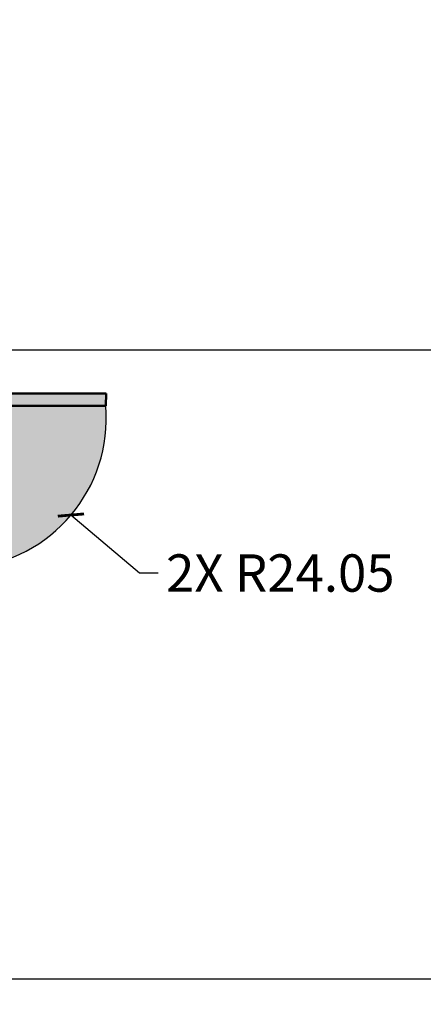
# Model space of a CAD drawing. Units: inches. Extents: x 925 to 2834, y 111 to 1355.
# Tile 11 of 25: x 1721 to 1785, y 723 to 882. Entities that reach past the tile are written whole.
import ezdxf

# ---------------------------------------------------------------- set-up
doc = ezdxf.new("R2010")
doc.units = ezdxf.units.IN
doc.header["$MEASUREMENT"] = 0
for name, color, linetype, lineweight in [('A-ANNO-DIMS', 2, 'Continuous', 18), ('A-DOOR', 2, 'Continuous', 25), ('A-FLOR-PATT', 252, 'Continuous', 13), ('A-WALL', 7, 'Continuous', 50)]:
    doc.layers.add(name, color=color, linetype=linetype, lineweight=lineweight)
doc.styles.get("Standard").update_dxf_attribs({"font": 'arial.ttf'})
doc.dimstyles.get("Standard").update_dxf_attribs({"dimtxt": 6, "dimasz": 3, "dimexe": 0.18, "dimexo": 0.0625, "dimgap": 0.09, "dimtad": 0, "dimtih": 1, "dimtoh": 1, "dimdec": 1, "dimzin": 0, "dimdsep": 46, "dimlunit": 3, "dimtxsty": 'Standard', "dimblk": 'ARCHTICK', "dimcen": 0.09, "dimadec": 0, "dimazin": 0, "dimtfac": 1, "dimtdec": 1, "dimtofl": 0, "dimtmove": 0, "dimatfit": 3, "dimfxl": 1, "dimtolj": 1, "dimtzin": 0, "dimarcsym": 0})

# ---------------------------------------------------------------- blocks, each defined once
blk = doc.blocks.new('_ArchTick')
at = {"color": 0, "linetype": 'ByBlock', "const_width": 0.15}
blk.add_lwpolyline([(-0.5, -0.5), (0.5, 0.5)], dxfattribs=at)
blk = doc.blocks.new('*D45')
at = {"layer": 'A-ANNO-DIMS', "color": 0, "lineweight": -2, "transparency": 16777216}
for p, q in [((1708.78, 727.59), (1988.62, 727.59)), ((1988.44, 727.59), (1988.44, 687.74)), ((1988.44, 641.59), (1988.44, 681.44)), ((1708.78, 641.59), (1988.62, 641.59))]:
    blk.add_line(p, q, dxfattribs=at)
at = {"layer": 'Defpoints', "color": 0, "transparency": 16777216}
for p in [(1708.71, 727.59), (1988.44, 727.59), (1708.71, 641.59)]:
    blk.add_point(p, dxfattribs=at)
at = {"layer": 'A-ANNO-DIMS', "color": 0, "lineweight": -2, "transparency": 16777216, "xscale": 3, "yscale": 3, "zscale": 3}
for p, rotation in [((1988.44, 727.59), 90), ((1988.44, 641.59), 270)]:
    blk.add_blockref('_ArchTick', p, dxfattribs=dict(at, rotation=rotation))
at = {"layer": 'A-ANNO-DIMS', "color": 0, "transparency": 16777216, "insert": (1988.44, 684.59), "char_height": 6, "attachment_point": 5}
blk.add_mtext('\\A1;86', dxfattribs=at)
blk = doc.blocks.new('*D46')
at = {"layer": 'A-ANNO-DIMS', "color": 0, "lineweight": -2, "transparency": 16777216}
for p, q in [((1708.78, 828.59), (1988.62, 828.59)), ((1988.44, 828.59), (1988.44, 781.24)), ((1988.44, 727.59), (1988.44, 774.94)), ((1708.78, 727.59), (1988.62, 727.59))]:
    blk.add_line(p, q, dxfattribs=at)
at = {"layer": 'Defpoints', "color": 0, "transparency": 16777216}
for p in [(1708.71, 828.59), (1988.44, 828.59), (1708.71, 727.59)]:
    blk.add_point(p, dxfattribs=at)
at = {"layer": 'A-ANNO-DIMS', "color": 0, "lineweight": -2, "transparency": 16777216, "xscale": 3, "yscale": 3, "zscale": 3}
for p, rotation in [((1988.44, 828.59), 90), ((1988.44, 727.59), 270)]:
    blk.add_blockref('_ArchTick', p, dxfattribs=dict(at, rotation=rotation))
at = {"layer": 'A-ANNO-DIMS', "color": 0, "transparency": 16777216, "insert": (1988.44, 778.09), "char_height": 6, "attachment_point": 5}
blk.add_mtext('\\A1;101', dxfattribs=at)
blk = doc.blocks.new('*D47')
at = {"layer": 'A-ANNO-DIMS', "color": 0, "lineweight": -2, "transparency": 16777216}
for p, q in [((1708.78, 903.59), (1988.62, 903.59)), ((1988.44, 903.59), (1988.44, 869.23)), ((1988.44, 828.59), (1988.44, 862.95)), ((1708.78, 828.59), (1988.62, 828.59))]:
    blk.add_line(p, q, dxfattribs=at)
at = {"layer": 'Defpoints', "color": 0, "transparency": 16777216}
for p in [(1708.71, 903.59), (1988.44, 903.59), (1708.71, 828.59)]:
    blk.add_point(p, dxfattribs=at)
at = {"layer": 'A-ANNO-DIMS', "color": 0, "lineweight": -2, "transparency": 16777216, "xscale": 3, "yscale": 3, "zscale": 3}
for p, rotation in [((1988.44, 903.59), 90), ((1988.44, 828.59), 270)]:
    blk.add_blockref('_ArchTick', p, dxfattribs=dict(at, rotation=rotation))
at = {"layer": 'A-ANNO-DIMS', "color": 0, "transparency": 16777216, "insert": (1988.44, 866.09), "char_height": 6, "attachment_point": 5}
blk.add_mtext('\\A1;75', dxfattribs=at)
blk = doc.blocks.new('*D82')
at = {"layer": 'A-ANNO-DIMS', "color": 0, "lineweight": -2, "transparency": 16777216}
for p, q in [((1710.32, 817.55), (1710.5, 817.55)), ((1710.41, 817.46), (1710.41, 817.64)), ((1739.82, 792.74), (1728.79, 802.05)), ((1742.82, 792.74), (1739.82, 792.74))]:
    blk.add_line(p, q, dxfattribs=at)
at = {"layer": 'Defpoints', "color": 0, "transparency": 16777216}
for p in [(1710.41, 817.55), (1728.79, 802.05)]:
    blk.add_point(p, dxfattribs=at)
at = {"layer": 'A-ANNO-DIMS', "color": 0, "lineweight": -2, "transparency": 16777216, "xscale": 3, "yscale": 3, "zscale": 3, "rotation": 139.8500923460391}
blk.add_blockref('_ArchTick', (1728.79, 802.05), dxfattribs=at)
at = {"layer": 'A-ANNO-DIMS', "color": 0, "transparency": 16777216, "insert": (1762.43, 792.74), "char_height": 6, "attachment_point": 5}
blk.add_mtext('\\A1;2X R24.05', dxfattribs=at)

msp = doc.modelspace()

# ---------------------------------------------------------------- hatches: boundary and pattern name
at = {"layer": 'A-FLOR-PATT', "transparency": 33554605}
h = msp.add_hatch(color=256, dxfattribs=at)
h.dxf.hatch_style = 1
h.paths.add_polyline_path([(1931.688, 1294.5638), (991.7375, 1294.5638), (991.7375, 172.1134), (1931.688, 172.1134)])
h.paths.add_polyline_path([(1910.7128, 1273.5886), (1910.7128, 193.0886), (1012.7128, 193.0886), (1012.7128, 1273.5886)], flags=16)
h.paths.add_polyline_path([(1850.7128, 1213.5886), (1850.7128, 253.0886), (1072.7128, 253.0886), (1072.7128, 1213.5886)], flags=0)
h.paths.add_polyline_path([(1838.7128, 1201.5886), (1838.7128, 265.0886), (1084.7128, 265.0886), (1084.7128, 530.5886), (1084.7128, 1201.5886)], flags=0)
h.paths.add_polyline_path([(1547.6758, 1155.7396), (1547.6758, 1119.115), (1513.0687, 1119.115), (1513.0687, 1155.7396)], flags=0)
h.paths.add_polyline_path([(1600.1067, 1154.9439), (1634.7139, 1154.9439), (1634.7139, 1119.115), (1600.1067, 1119.115)], flags=0)
h.paths.add_polyline_path([(1505.2502, 1144.5358), (1505.2502, 1119.115), (1470.643, 1119.115), (1470.643, 1144.5358)], flags=0)
h.paths.add_polyline_path([(1559.1357, 1141.0962), (1593.7428, 1141.0962), (1593.7428, 1119.115), (1559.1357, 1119.115)], flags=0)
h.paths.add_polyline_path([(1462.8966, 1154.9439), (1462.8966, 1119.115), (1428.2895, 1119.115), (1428.2895, 1154.9439)], flags=0)
h.paths.add_polyline_path([(1642.4603, 1144.5358), (1677.0675, 1144.5358), (1677.0675, 1119.115), (1642.4603, 1119.115)], flags=0)
h.paths.add_polyline_path([(1422.3508, 1141.0962), (1422.3508, 1119.115), (1387.7436, 1119.115), (1387.7436, 1141.0962)], flags=0)
h.paths.add_polyline_path([(1684.8859, 1155.7396), (1719.4931, 1155.7396), (1719.4931, 1119.115), (1684.8859, 1119.115)], flags=0)
h.paths.add_polyline_path([(1718.7128, 1081.5886), (1718.7128, 1050.1249), (1715.7128, 1050.1249), (1715.7128, 1026.1249), (1715.7128, 1002.1249), (1718.7128, 1002.1249), (1730.7128, 1002.1249), (1730.7128, 998.1249), (1730.7128, 990.1249), (1730.7128, 986.1249), (1718.7128, 986.1249), (1718.7128, 893.5886), (1715.3735, 893.5886), (1715.3735, 891.5886), (1713.3735, 891.5886, 0.41421356), (1677.3735, 855.5886), (1713.3735, 855.5886), (1713.3735, 853.5886), (1715.3735, 853.5886), (1715.3735, 851.5886), (1718.7128, 851.5886), (1718.7128, 821.5865), (1734.4655, 821.5865), (1734.3735, 819.5886, -0.41421356), (1712.4415, 793.5886), (1712.4415, 791.5886), (1718.7128, 791.5886), (1718.7128, 717.5886), (1718.7128, 669.5886), (1732.7128, 669.5886), (1732.7128, 665.5886), (1732.7128, 641.5886), (1732.7128, 634.5886), (1732.7128, 610.5886), (1732.7128, 603.5886), (1718.7128, 603.5886), (1718.7128, 385.0886), (1434.2128, 385.0886), (1434.2128, 530.5886), (1410.2128, 530.5886), (1408.2128, 530.5886), (1408.2128, 532.5886, 0.41421356), (1372.2128, 568.5886), (1372.2128, 532.5886), (1370.2128, 532.5886), (1370.2128, 530.5886), (1368.2128, 530.5886), (1282.2128, 530.5886), (1210.2128, 530.5886), (1200.2128, 530.5886), (1200.2128, 542.1915), (1183.2307, 542.1915), (1183.2307, 546.1915), (1200.2128, 546.1915), (1200.2128, 572.1915), (1183.2307, 572.1915), (1183.2307, 576.1915), (1200.2128, 576.1915), (1200.2128, 727.5886), (1210.2128, 727.5886), (1234.2128, 727.5886), (1259.7128, 727.5886), (1259.7128, 775.5886), (1259.7128, 799.5886), (1259.7128, 847.5886), (1259.7128, 993.5872), (1259.7128, 1065.5872), (1259.7128, 1071.5886), (1219.6318, 1071.5886), (1219.6318, 1081.5886), (1084.7128, 1081.5886), (1084.7128, 1119.115), (1256.8974, 1119.115), (1256.8974, 1154.9439), (1291.5046, 1154.9439), (1291.5046, 1119.115), (1256.8974, 1119.115), (1256.6723, 1081.5886), (1293.7128, 1081.5886), (1341.7128, 1081.5886), (1341.7128, 1093.5886), (1347.7128, 1093.5886), (1371.7128, 1093.5886), (1377.7128, 1093.5886), (1377.7128, 1081.5886), (1668.7128, 1081.5886), (1668.7128, 1117.5886), (1675.7128, 1117.5886), (1711.7128, 1117.5886), (1718.7128, 1117.5886)], flags=0)
h.paths.add_polyline_path([(1376.2838, 1155.7396), (1376.2838, 1119.115), (1341.6766, 1119.115), (1341.6766, 1155.7396)], flags=0)
h.paths.add_polyline_path([(1341.7128, 1076.0886), (1293.7128, 1076.0886), (1293.7128, 1071.5886), (1269.7128, 1071.5886), (1269.7128, 1065.5872), (1266.7128, 1065.5872), (1266.7128, 1029.5872), (1265.7128, 1029.5872), (1265.7128, 993.5872), (1269.7128, 993.5872), (1269.7128, 903.5886), (1269.7128, 893.5886), (1269.7128, 847.5886), (1265.2128, 847.5886), (1265.2128, 799.5886), (1269.7128, 799.5886), (1269.7128, 775.5886), (1265.2128, 775.5886), (1265.2128, 727.5886), (1269.7128, 727.5886), (1444.2128, 727.5886), (1444.2128, 717.5886), (1234.2128, 717.5886), (1234.2128, 722.0886), (1210.2128, 722.0886), (1210.2128, 717.5886), (1210.2128, 540.5886), (1210.2128, 536.0886), (1282.2128, 536.0886), (1282.2128, 535.0886), (1210.2128, 535.0886), (1210.2128, 540.5886), (1210.2128, 717.5886), (1210.2128, 723.0886), (1234.2128, 723.0886), (1234.2128, 717.5886), (1444.2128, 717.5886), (1444.2128, 727.5886), (1269.7128, 727.5886), (1264.2128, 727.5886), (1264.2128, 775.5886), (1269.7128, 775.5886), (1269.7128, 799.5886), (1264.2128, 799.5886), (1264.2128, 847.5886), (1269.7128, 847.5886), (1269.7128, 893.5886), (1269.7128, 903.5886), (1269.7128, 993.5872), (1264.7128, 993.5872), (1264.7128, 1029.5872), (1265.7128, 1029.5872), (1265.7128, 1065.5872), (1269.7128, 1065.5872), (1269.7128, 1071.5886), (1293.7128, 1071.5886), (1293.7128, 1077.0886), (1341.7128, 1077.0886)], flags=0)
h.paths.add_polyline_path([(1730.9529, 1141.0962), (1765.5601, 1141.0962), (1765.5601, 1119.115), (1730.9529, 1119.115)], flags=0)
h.paths.add_polyline_path([(1333.8582, 1144.5358), (1333.8582, 1119.115), (1299.251, 1119.115), (1299.251, 1144.5358)], flags=0)
h.paths.add_polyline_path([(1592.7128, 968.5886), (1596.0342, 968.5886), (1602.7128, 968.5886), (1708.7128, 968.5886), (1708.7128, 903.5886), (1602.7128, 903.5886), (1602.7128, 938.5886), (1592.7128, 938.5886), (1592.7128, 903.5886), (1451.7128, 903.5886), (1451.7128, 893.5886), (1511.7128, 893.5886), (1511.7128, 881.5886), (1515.2128, 881.5886), (1518.7128, 881.5886), (1518.7128, 893.5886), (1592.7128, 893.5886), (1592.7128, 799.5886), (1518.7128, 799.5886), (1518.7128, 857.5886), (1511.7128, 857.5886), (1511.7128, 799.5886), (1511.7128, 772.0886), (1521.7128, 772.0886), (1521.7128, 792.5886), (1592.7128, 792.5886), (1592.7128, 727.5886), (1521.7128, 727.5886), (1521.7128, 748.0886), (1511.7128, 748.0886), (1511.7128, 717.5886), (1708.7128, 717.5886), (1714.2128, 717.5886), (1714.2128, 669.5886), (1708.7128, 669.5886), (1708.7128, 641.5886), (1492.2128, 641.5886), (1492.2128, 631.5886), (1621.2128, 631.5886), (1621.2128, 443.0886), (1625.7128, 443.0886), (1625.7128, 503.0886), (1625.7128, 507.5886), (1625.7128, 631.5886), (1708.7128, 631.5886), (1708.7128, 507.5886), (1655.7128, 507.5886), (1655.7128, 503.0886), (1708.7128, 503.0886), (1708.7128, 395.0886), (1625.7128, 395.0886), (1625.7128, 419.0886), (1621.2128, 419.0886), (1621.2128, 395.0886), (1482.2128, 395.0886), (1482.2128, 385.0886), (1434.2128, 385.0886), (1434.2128, 433.0886), (1444.2128, 433.0886), (1444.2128, 631.5886), (1450.2128, 631.5886), (1450.2128, 634.91), (1452.2128, 634.91), (1452.2128, 669.5886), (1454.2128, 669.5886, -0.40021217), (1490.1712, 635.3173), (1492.2128, 635.3173), (1492.2128, 641.5886), (1564.7128, 641.5886), (1564.7128, 677.5886), (1672.7128, 677.5886), (1672.7128, 681.5886), (1564.7128, 681.5886), (1564.7128, 717.5886), (1511.7128, 717.5886), (1511.7128, 748.0886), (1511.7128, 772.0886), (1511.7128, 799.5886), (1511.7128, 857.5886), (1511.8913, 857.5886), (1511.8913, 859.5886), (1515.6201, 859.5886, 0.41421356), (1537.552, 879.5886), (1513.552, 879.5886), (1511.8913, 879.5886), (1511.8913, 881.5886), (1511.7128, 881.5886), (1511.7128, 893.5886), (1451.7128, 893.5886), (1451.7128, 903.5886), (1592.7128, 903.5886), (1592.7128, 938.5886), (1592.7128, 940.5886), (1596.4415, 940.5886, 0.41421356), (1618.3735, 966.5886), (1594.3735, 966.5886), (1592.7128, 966.5886)], flags=0)
h.paths.add_polyline_path([(1377.7128, 903.5886), (1377.7128, 893.5886), (1305.7128, 893.5886), (1305.7128, 903.5886)], flags=0)
h.paths.add_polyline_path([(1708.7128, 821.5886), (1712.0342, 821.5886), (1712.0342, 819.5886), (1710.3735, 819.5886), (1708.7128, 819.5886)], flags=0)
h.paths.add_polyline_path([(1576.7128, 695.1992), (1575.5896, 693.6649), (1575.9687, 694.6994), (1575.4438, 695.1992), (1575.9687, 695.699), (1575.5896, 696.7335)], flags=0)
h.paths.add_polyline_path([(1565.9817, 662.3134), (1565.4568, 661.8136), (1565.8359, 660.7791), (1564.7128, 662.3134), (1565.8359, 663.8477), (1565.4568, 662.8132)], flags=0)
h.paths.add_polyline_path([(1444.2128, 433.0886), (1444.2128, 395.0886), (1482.2128, 395.0886), (1482.2128, 389.0886), (1438.2128, 389.0886), (1438.2128, 391.8608), (1438.2128, 433.0886)], flags=0)
h.paths.add_polyline_path([(1410.2128, 506.5886), (1410.2128, 289.0886), (1108.7128, 289.0886), (1108.7128, 506.5886)], flags=0)
h.paths.add_polyline_path([(1612.3153, 838.3016), (1680.4151, 838.3016), (1680.4151, 851.3131), (1612.3153, 851.3131)], flags=8)
h.paths.add_polyline_path([(1208.3174, 395.0436), (1282.1017, 395.0436), (1282.1017, 408.0552), (1208.3174, 408.0552)], flags=8)
h.paths.add_polyline_path([(1291.8049, 598.7427), (1369.8017, 598.7427), (1369.8017, 611.7542), (1291.8049, 611.7542)], flags=8)
h.paths.add_polyline_path([(1119.679, 917.3022), (1191.0817, 917.3022), (1191.0817, 930.3137), (1119.679, 930.3137)], flags=8)
h.paths.add_polyline_path([(1332.2261, 815.9808), (1410.2258, 815.9808), (1410.2258, 829.001), (1332.2261, 829.001)], flags=8)
h.paths.add_polyline_path([(1390.9013, 955.8158), (1475.4981, 955.8158), (1475.4981, 968.8273), (1390.9013, 968.8273)], flags=8)
h.paths.add_polyline_path([(1620.3436, 998.9325), (1688.4434, 998.9325), (1688.4434, 1011.944), (1620.3436, 1011.944)], flags=8)
h.paths.add_polyline_path([(1620.3436, 914.1039), (1691.7405, 914.1039), (1691.7405, 927.1155), (1620.3436, 927.1155)], flags=8)
h.paths.add_polyline_path([(1521.4542, 816.005), (1589.5569, 816.005), (1589.5569, 829.0253), (1521.4542, 829.0253)], flags=8)
h.paths.add_polyline_path([(1528.524, 740.3497), (1602.3082, 740.3497), (1602.3082, 753.3613), (1528.524, 753.3613)], flags=8)
h.paths.add_polyline_path([(1627.6094, 762.6128), (1702.3091, 762.6128), (1702.3091, 775.6244), (1627.6094, 775.6244)], flags=8)
h.paths.add_polyline_path([(1610.5442, 657.2751), (1684.3284, 657.2751), (1684.3284, 670.2867), (1610.5442, 670.2867)], flags=8)
h.paths.add_polyline_path([(1636.6983, 519.472), (1711.3981, 519.472), (1711.3981, 532.4835), (1636.6983, 532.4835)], flags=8)
h.paths.add_polyline_path([(1616.8577, 424.8539), (1694.8545, 424.8539), (1694.8545, 437.8654), (1616.8577, 437.8654)], flags=8)
h.paths.add_polyline_path([(1506.1456, 460.8838), (1579.9299, 460.8838), (1579.9299, 473.8953), (1506.1456, 473.8953)], flags=8)
h.paths.add_polyline_path([(1624.6119, 784.6011), (1696.9185, 784.6011), (1696.9185, 797.7864), (1624.6119, 797.7864)], flags=8)
h.paths.add_polyline_path([(1606.3732, 854.2194), (1683.3039, 854.2194), (1683.3039, 867.4048), (1606.3732, 867.4048)], flags=8)
h.paths.add_polyline_path([(1127.8008, 940.3581), (1165.1637, 940.3581), (1165.1637, 953.5348), (1127.8008, 953.5348)], flags=8)
h.paths.add_polyline_path([(1620.8657, 1019.4968), (1677.3447, 1019.4968), (1677.3447, 1032.6735), (1620.8657, 1032.6735)], flags=8)
h.paths.add_polyline_path([(1620.8643, 930.1821), (1703.0564, 930.1821), (1703.0564, 943.3675), (1620.8643, 943.3675)], flags=8)
h.paths.add_polyline_path([(1324.5702, 836.8338), (1408.0892, 836.8338), (1408.0892, 850.0191), (1324.5702, 850.0191)], flags=8)
h.paths.add_polyline_path([(1281.6584, 622.8885), (1383.6213, 622.8885), (1383.6213, 636.0739), (1281.6584, 636.0739)], flags=8)
h.paths.add_polyline_path([(1210.6721, 416.7893), (1269.1299, 416.7893), (1269.1299, 429.9747), (1210.6721, 429.9747)], flags=8)
h.paths.add_polyline_path([(1507.8264, 477.4836), (1586.7329, 477.4836), (1586.7329, 490.669), (1507.8264, 490.669)], flags=8)
h.paths.add_polyline_path([(1643.6238, 443.8135), (1696.6696, 443.8135), (1696.6696, 456.5643), (1643.6238, 456.5643)], flags=8)
h.paths.add_polyline_path([(1647.2466, 540.5638), (1693.1825, 540.5638), (1693.1825, 553.7491), (1647.2466, 553.7491)], flags=8)
h.paths.add_polyline_path([(1626.0633, 668.5064), (1673.3174, 668.5064), (1673.3174, 681.6831), (1626.0633, 681.6831)], flags=8)
h.paths.add_polyline_path([(1538.2915, 830.7872), (1567.5942, 830.7872), (1567.5942, 843.5293), (1538.2915, 843.5293)], flags=8)
h.paths.add_polyline_path([(1530.9338, 754.0477), (1559.576, 754.0477), (1559.576, 766.7898), (1530.9338, 766.7898)], flags=8)
h.paths.add_polyline_path([(1351.2461, 979.2309), (1513.8919, 979.2309), (1513.8919, 992.4076), (1351.2461, 992.4076)], flags=8)
at = {"layer": 'A-FLOR-PATT'}
h = msp.add_hatch(color=256, dxfattribs=at)
h.dxf.hatch_style = 1
h.paths.add_polyline_path([(1850.7128, 1213.5886), (1072.7128, 1213.5886), (1072.7128, 253.0886), (1850.7128, 253.0886)])
h.paths.add_polyline_path([(1084.7128, 1201.5886), (1838.7128, 1201.5886), (1838.7128, 265.0886), (1084.7128, 265.0886)], flags=16)
h.paths.add_polyline_path([(1183.2307, 576.1915), (1200.2128, 576.1915), (1200.2128, 727.5886), (1210.2128, 727.5886), (1234.2128, 727.5886), (1259.7128, 727.5886), (1259.7128, 775.5886), (1259.7128, 799.5886), (1259.7128, 847.5886), (1259.7128, 993.5872), (1259.7128, 1065.5872), (1259.7128, 1071.5886), (1219.6318, 1071.5886), (1219.6318, 1081.5886), (1293.7128, 1081.5886), (1341.7128, 1081.5886), (1341.7128, 1093.5886), (1347.7128, 1093.5886), (1347.7128, 1081.5886), (1371.7128, 1081.5886), (1371.7128, 1093.5886), (1377.7128, 1093.5886), (1377.7128, 1081.5886), (1668.7128, 1081.5886), (1668.7128, 1117.5886), (1675.7128, 1117.5886), (1675.7128, 1081.5886), (1711.7128, 1081.5886), (1711.7128, 1117.5886), (1718.7128, 1117.5886), (1718.7128, 1081.5886), (1718.7128, 1050.1249), (1715.7128, 1050.1249), (1715.7128, 1026.1249), (1715.7128, 1002.1249), (1718.7128, 1002.1249), (1730.7128, 1002.1249), (1730.7128, 998.1249), (1730.7128, 990.1249), (1730.7128, 986.1249), (1718.7128, 986.1249), (1718.7128, 893.5886), (1715.3735, 893.5886), (1715.3735, 891.5886), (1713.3735, 891.5886, 0.41421356), (1677.3735, 855.5886), (1713.3735, 855.5886), (1713.3735, 853.5886), (1715.3735, 853.5886), (1715.3735, 851.5886), (1718.7128, 851.5886), (1718.7128, 821.5865), (1734.4655, 821.5865), (1734.3735, 819.5886, -0.41421356), (1712.4415, 793.5886), (1712.4415, 791.5886), (1718.7128, 791.5886), (1718.7128, 717.5886), (1718.7128, 669.5886), (1732.7128, 669.5886), (1732.7128, 665.5886), (1732.7128, 641.5886), (1732.7128, 634.5886), (1732.7128, 610.5886), (1732.7128, 603.5886), (1718.7128, 603.5886), (1718.7128, 385.0886), (1434.2128, 385.0886), (1434.2128, 433.0886), (1434.2128, 530.5886), (1410.2128, 530.5886), (1408.2128, 530.5886), (1408.2128, 532.5886, 0.41421356), (1372.2128, 568.5886), (1372.2128, 532.5886), (1370.2128, 532.5886), (1370.2128, 530.5886), (1368.2128, 530.5886), (1282.2128, 530.5886), (1210.2128, 530.5886), (1200.2128, 530.5886), (1200.2128, 542.1915), (1183.2307, 542.1915), (1183.2307, 546.1915), (1200.2128, 546.1915), (1200.2128, 572.1915), (1183.2307, 572.1915)], flags=0)
h.paths.add_polyline_path([(1210.2128, 717.5886), (1210.2128, 723.0886), (1234.2128, 723.0886), (1234.2128, 717.5886), (1444.2128, 717.5886), (1444.2128, 727.5886), (1269.7128, 727.5886), (1264.2128, 727.5886), (1264.2128, 775.5886), (1269.7128, 775.5886), (1269.7128, 799.5886), (1264.2128, 799.5886), (1264.2128, 847.5886), (1269.7128, 847.5886), (1269.7128, 893.5886), (1269.7128, 903.5886), (1269.7128, 993.5872), (1264.7128, 993.5872), (1264.7128, 1029.5872), (1265.7128, 1029.5872), (1265.7128, 1065.5872), (1269.7128, 1065.5872), (1269.7128, 1071.5886), (1293.7128, 1071.5886), (1293.7128, 1077.0886), (1341.7128, 1077.0886), (1341.7128, 1076.0886), (1293.7128, 1076.0886), (1293.7128, 1071.5886), (1269.7128, 1071.5886), (1269.7128, 1065.5872), (1266.7128, 1065.5872), (1266.7128, 1029.5872), (1265.7128, 1029.5872), (1265.7128, 993.5872), (1269.7128, 993.5872), (1269.7128, 903.5886), (1269.7128, 893.5886), (1269.7128, 847.5886), (1265.2128, 847.5886), (1265.2128, 799.5886), (1269.7128, 799.5886), (1269.7128, 775.5886), (1265.2128, 775.5886), (1265.2128, 727.5886), (1269.7128, 727.5886), (1444.2128, 727.5886), (1444.2128, 717.5886), (1234.2128, 717.5886), (1234.2128, 722.0886), (1210.2128, 722.0886), (1210.2128, 717.5886), (1210.2128, 540.5886), (1210.2128, 536.0886), (1282.2128, 536.0886), (1282.2128, 535.0886), (1210.2128, 535.0886), (1210.2128, 540.5886)], flags=0)
h.paths.add_polyline_path([(1450.2128, 634.91), (1452.2128, 634.91), (1452.2128, 669.5886), (1454.2128, 669.5886, -0.40021217), (1490.1712, 635.3173), (1492.2128, 635.3173), (1492.2128, 641.5886), (1564.7128, 641.5886), (1564.7128, 677.5886), (1672.7128, 677.5886), (1672.7128, 681.5886), (1564.7128, 681.5886), (1564.7128, 717.5886), (1511.7128, 717.5886), (1511.7128, 748.0886), (1511.7128, 772.0886), (1511.7128, 799.5886), (1511.7128, 857.5886), (1511.8913, 857.5886), (1511.8913, 859.5886), (1515.6201, 859.5886, 0.41421356), (1537.552, 879.5886), (1513.552, 879.5886), (1511.8913, 879.5886), (1511.8913, 881.5886), (1511.7128, 881.5886), (1511.7128, 893.5886), (1451.7128, 893.5886), (1451.7128, 903.5886), (1592.7128, 903.5886), (1592.7128, 938.5886), (1592.7128, 940.5886), (1596.4415, 940.5886, 0.41421356), (1618.3735, 966.5886), (1594.3735, 966.5886), (1592.7128, 966.5886), (1592.7128, 968.5886), (1596.0342, 968.5886), (1602.7128, 968.5886), (1708.7128, 968.5886), (1708.7128, 903.5886), (1602.7128, 903.5886), (1602.7128, 938.5886), (1592.7128, 938.5886), (1592.7128, 903.5886), (1451.7128, 903.5886), (1451.7128, 893.5886), (1511.7128, 893.5886), (1511.7128, 881.5886), (1518.7128, 881.5886), (1518.7128, 893.5886), (1592.7128, 893.5886), (1592.7128, 799.5886), (1518.7128, 799.5886), (1518.7128, 857.5886), (1511.7128, 857.5886), (1511.7128, 799.5886), (1511.7128, 772.0886), (1521.7128, 772.0886), (1521.7128, 792.5886), (1592.7128, 792.5886), (1592.7128, 727.5886), (1521.7128, 727.5886), (1521.7128, 748.0886), (1511.7128, 748.0886), (1511.7128, 717.5886), (1708.7128, 717.5886), (1714.2128, 717.5886), (1714.2128, 669.5886), (1708.7128, 669.5886), (1708.7128, 641.5886), (1492.2128, 641.5886), (1492.2128, 631.5886), (1621.2128, 631.5886), (1621.2128, 443.0886), (1625.7128, 443.0886), (1625.7128, 503.0886), (1625.7128, 507.5886), (1625.7128, 631.5886), (1708.7128, 631.5886), (1708.7128, 507.5886), (1655.7128, 507.5886), (1655.7128, 503.0886), (1708.7128, 503.0886), (1708.7128, 395.0886), (1625.7128, 395.0886), (1625.7128, 419.0886), (1621.2128, 419.0886), (1621.2128, 395.0886), (1482.2128, 395.0886), (1482.2128, 389.0886), (1438.2128, 389.0886), (1438.2128, 391.8608), (1438.2128, 433.0886), (1444.2128, 433.0886), (1444.2128, 631.5886), (1450.2128, 631.5886)], flags=0)
h.paths.add_polyline_path([(1444.2128, 433.0886), (1444.2128, 395.0886), (1482.2128, 395.0886), (1482.2128, 391.0886), (1440.2128, 391.0886), (1440.2128, 391.8608), (1440.2128, 433.0886)], flags=0)
h.paths.add_polyline_path([(1305.7128, 893.5886), (1305.7128, 903.5886), (1377.7128, 903.5886), (1377.7128, 893.5886)], flags=0)
h.paths.add_polyline_path([(1564.7128, 662.3134), (1565.8359, 663.8477), (1565.4568, 662.8132), (1565.9817, 662.3134), (1565.4568, 661.8136), (1565.8359, 660.7791)], flags=0)
h.paths.add_polyline_path([(1575.4438, 695.1992), (1575.9687, 695.699), (1575.5896, 696.7335), (1576.7128, 695.1992), (1575.5896, 693.6649), (1575.9687, 694.6994)], flags=0)
h.paths.add_polyline_path([(1708.7128, 821.5886), (1712.0342, 821.5886), (1712.0342, 819.5886), (1710.3735, 819.5886), (1708.7128, 819.5886)], flags=0)
at = {"layer": 'A-FLOR-PATT', "transparency": 33554605}
h = msp.add_hatch(color=256, dxfattribs=at)
h.dxf.hatch_style = 1
h.paths.add_polyline_path([(1708.7128, 791.5886), (1708.7128, 793.5886), (1712.4415, 793.5886, 0.41421356), (1734.3735, 819.5886), (1710.3735, 819.5886), (1708.7128, 819.5886), (1708.7128, 821.5886), (1602.7128, 821.5886), (1602.7128, 727.5886), (1708.7128, 727.5886)])
h.paths.add_polyline_path([(1708.7128, 851.5886), (1712.052, 851.5886), (1712.052, 853.5886), (1677.3735, 853.5886), (1677.3735, 855.5886, -0.40021217), (1711.6447, 891.5471), (1711.6447, 893.5886), (1708.7128, 893.5886), (1602.7128, 893.5886), (1602.7128, 828.5886), (1708.7128, 828.5886)])
h.paths.add_polyline_path([(1708.7128, 968.5886), (1618.4656, 968.5886), (1618.3735, 966.5886, -0.41421356), (1596.4415, 940.5886), (1596.4415, 938.5886), (1602.7128, 938.5886), (1602.7128, 903.5886), (1708.7128, 903.5886)])
h.paths.add_polyline_path([(1708.7128, 717.5886), (1672.7128, 717.5886), (1672.7128, 641.5886), (1708.7128, 641.5886)])
h.paths.add_polyline_path([(1588.7128, 717.5886), (1576.7128, 717.5886), (1576.7128, 681.5886), (1588.7128, 681.5886)])
h.paths.add_polyline_path([(1576.7128, 717.5886), (1564.7128, 717.5886), (1564.7128, 695.1992), (1575.4438, 695.1992), (1575.9687, 695.699), (1575.5896, 696.7335), (1576.7128, 695.1992)])
h.paths.add_polyline_path([(1576.7128, 695.1992), (1575.5896, 693.6649), (1575.9687, 694.6994), (1575.4438, 695.1992), (1564.7128, 695.1992), (1564.7128, 681.5886), (1576.7128, 681.5886)])
h.paths.add_polyline_path([(1600.7128, 717.5886), (1588.7128, 717.5886), (1588.7128, 681.5886), (1600.7128, 681.5886)])
h.paths.add_polyline_path([(1612.7128, 717.5886), (1600.7128, 717.5886), (1600.7128, 681.5886), (1612.7128, 681.5886)])
h.paths.add_polyline_path([(1624.7128, 717.5886), (1612.7128, 717.5886), (1612.7128, 681.5886), (1624.7128, 681.5886)])
h.paths.add_polyline_path([(1636.7128, 717.5886), (1624.7128, 717.5886), (1624.7128, 681.5886), (1636.7128, 681.5886)])
h.paths.add_polyline_path([(1648.7128, 717.5886), (1636.7128, 717.5886), (1636.7128, 681.5886), (1648.7128, 681.5886)])
h.paths.add_polyline_path([(1660.7128, 717.5886), (1648.7128, 717.5886), (1648.7128, 681.5886), (1660.7128, 681.5886)])
h.paths.add_polyline_path([(1672.7128, 717.5886), (1660.7128, 717.5886), (1660.7128, 681.5886), (1672.7128, 681.5886)])
h.paths.add_polyline_path([(1576.7128, 662.3134), (1565.9817, 662.3134), (1565.4568, 661.8136), (1565.8359, 660.7791), (1564.7128, 662.3134), (1564.7128, 641.5886), (1576.7128, 641.5886)])
h.paths.add_polyline_path([(1576.7128, 677.5886), (1564.7128, 677.5886), (1564.7128, 662.3134), (1565.8359, 663.8477), (1565.4568, 662.8132), (1565.9817, 662.3134), (1576.7128, 662.3134)])
h.paths.add_polyline_path([(1588.7128, 677.5886), (1576.7128, 677.5886), (1576.7128, 641.5886), (1588.7128, 641.5886)])
h.paths.add_polyline_path([(1600.7128, 677.5886), (1588.7128, 677.5886), (1588.7128, 641.5886), (1600.7128, 641.5886)])
h.paths.add_polyline_path([(1612.7128, 677.5886), (1600.7128, 677.5886), (1600.7128, 641.5886), (1612.7128, 641.5886)])
h.paths.add_polyline_path([(1624.7128, 677.5886), (1612.7128, 677.5886), (1612.7128, 641.5886), (1624.7128, 641.5886)])
h.paths.add_polyline_path([(1636.7128, 677.5886), (1624.7128, 677.5886), (1624.7128, 641.5886), (1636.7128, 641.5886)])
h.paths.add_polyline_path([(1648.7128, 677.5886), (1636.7128, 677.5886), (1636.7128, 641.5886), (1648.7128, 641.5886)])
h.paths.add_polyline_path([(1660.7128, 677.5886), (1648.7128, 677.5886), (1648.7128, 641.5886), (1660.7128, 641.5886)])
h.paths.add_polyline_path([(1672.7128, 677.5886), (1660.7128, 677.5886), (1660.7128, 641.5886), (1672.7128, 641.5886)])
h.paths.add_polyline_path([(1627.6094, 762.6128), (1702.3091, 762.6128), (1702.3091, 775.6244), (1627.6094, 775.6244)], flags=24)
h.paths.add_polyline_path([(1624.6119, 784.6011), (1696.9185, 784.6011), (1696.9185, 797.7864), (1624.6119, 797.7864)], flags=24)
h.paths.add_polyline_path([(1612.3153, 838.3016), (1680.4151, 838.3016), (1680.4151, 851.3131), (1612.3153, 851.3131)], flags=24)
h.paths.add_polyline_path([(1606.3732, 854.2194), (1683.3039, 854.2194), (1683.3039, 867.4048), (1606.3732, 867.4048)], flags=24)
h.paths.add_polyline_path([(1620.3436, 914.1039), (1691.7405, 914.1039), (1691.7405, 927.1155), (1620.3436, 927.1155)], flags=24)
h.paths.add_polyline_path([(1620.8643, 930.1821), (1703.0564, 930.1821), (1703.0564, 943.3675), (1620.8643, 943.3675)], flags=24)
h.paths.add_polyline_path([(1610.5442, 657.2751), (1684.3284, 657.2751), (1684.3284, 670.2867), (1610.5442, 670.2867)], flags=9)
h.paths.add_polyline_path([(1626.0633, 668.5064), (1673.3174, 668.5064), (1673.3174, 681.6831), (1626.0633, 681.6831)], flags=9)
at = {"layer": 'A-FLOR-PATT'}
h = msp.add_hatch(color=256, dxfattribs=at)
h.dxf.hatch_style = 1
h.paths.add_polyline_path([(1713.3735, 855.5886), (1677.3735, 855.5886), (1677.3735, 853.5886), (1713.3735, 853.5886)])
h.paths.add_polyline_path([(1372.2128, 568.5886), (1370.2128, 568.5886), (1370.2128, 532.5886), (1372.2128, 532.5886)])
h.paths.add_polyline_path([(1734.4655, 821.5865), (1712.0342, 821.5865), (1712.0342, 819.5886), (1734.3735, 819.5886)])
h.paths.add_polyline_path([(1454.2128, 669.5886), (1452.2128, 669.5886), (1452.2128, 633.5886), (1454.2128, 633.5886)])
h.paths.add_polyline_path([(1537.6441, 881.5865), (1515.2128, 881.5865), (1515.2128, 879.5886), (1537.552, 879.5886)])

# ---------------------------------------------------------------- linework, layer by layer
at = {"layer": 'A-DOOR'}
msp.add_arc((1710.4075, 817.5546), 24.0521, 274.851115, 4.851115, dxfattribs=at)
at = {"layer": 'A-WALL'}
for p, q in [((1734.4655, 821.5865), (1712.0342, 821.5865)), ((1718.7128, 821.5886), (1734.4655, 821.5865)), ((1734.3735, 819.5886), (1734.4655, 821.5865)), ((1710.3735, 819.5886), (1734.3735, 819.5886))]:
    msp.add_line(p, q, dxfattribs=at)

# ---------------------------------------------------------------- dimensions: what is measured, and where the dimension line sits
at = {"layer": 'A-ANNO-DIMS'}
for base, p1, p2, picture, middle in [((1988.438, 903.5886), (1708.7128, 828.5886), (1708.7128, 903.5886), '*D47', (1988.438, 866.0886)), ((1988.438, 828.5886), (1708.7128, 727.5886), (1708.7128, 828.5886), '*D46', (1988.438, 778.0886)), ((1988.438, 727.5886), (1708.7128, 641.5886), (1708.7128, 727.5886), '*D45', (1988.438, 684.5886))]:
    dim = msp.add_linear_dim(base=base, p1=p1, p2=p2, angle=90, dimstyle='Standard', override={"dimdec": 0, "dimlfac": 1, "dimrnd": 0, "dimzin": 0, "dimdsep": 46, "dimlunit": 2}, dxfattribs=at)
    dim.commit()
    dim.dimension.update_dxf_attribs({"geometry": picture, "text_midpoint": middle})
dim = msp.add_radius_dim(center=(1710.4075, 817.5546), mpoint=(1728.792, 802.046), text='2X <>', dimstyle='Standard', override={"dimdec": 2, "dimlfac": 1, "dimrnd": 0, "dimzin": 0, "dimdsep": 46, "dimlunit": 2}, dxfattribs=at)
dim.commit()
dim.dimension.update_dxf_attribs({"geometry": '*D82', "text_midpoint": (1762.427, 792.7409), "dimtype": 164})

doc.saveas('drawing.dxf')
